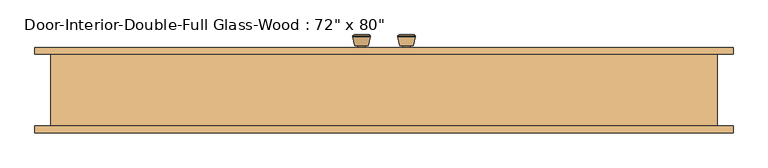
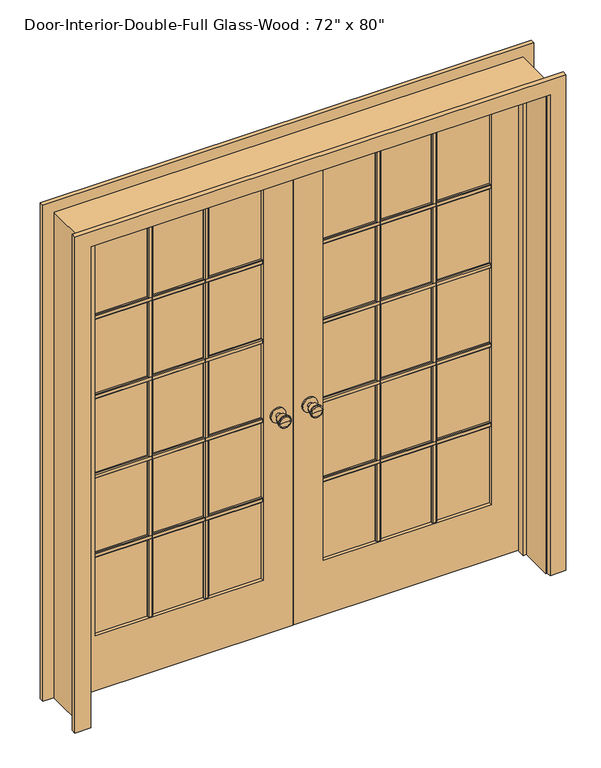
"""IFC4 building model written with IfcOpenShell, lengths in millimetres: door geometry."""

from ifc_helpers import new_model, si_unit, point, frame, frame_2d, origin, place, context, project, spatial, polyline, circle_curve, trimmed, segment, composite_curve, outline, extrude, faceted_brep, source, transform, mapped, element, save
from ifc_brep_helpers import plane_surface, cylinder_surface, revolved_surface, advanced_brep


def door_48c357d2(model_context):
    return source(origin(), model_context, "Body", "SolidModel", [
        advanced_brep(
        [(-63.5, 104.425, 914.4), (-73.5, 104.425, 914.4), (-53.5, 104.425, 914.4), (-83.9758676, 153.425, 914.4), (-63.5, 153.425, 914.4), (-43.0241324, 153.425, 914.4), (-88.5, 151.5971319, 914.4), (-38.5, 151.5971319, 914.4), (-88.5, 148.1334537, 914.4), (-38.5, 148.1334537, 914.4), (-82.136236, 123.425, 914.4), (-44.863764, 123.425, 914.4), (-73.5, 123.425, 914.4), (-53.5, 123.425, 914.4)],
        [
            (0, 1),
            (1, 2, circle_curve(frame((-63.5, 104.425, 914.4), z_axis=(0.0, -1.0, 0.0), x_axis=(1.0, 0.0, 0.0)), 10.0)),
            (2, 0),
            (2, 1, circle_curve(frame((-63.5, 104.425, 914.4), z_axis=(0.0, -1.0, 0.0), x_axis=(1.0, 0.0, 0.0)), 10.0)),
            (3, 4),
            (4, 5),
            (5, 3, circle_curve(frame((-63.5, 153.425, 914.4), z_axis=(0.0, 1.0, 0.0), x_axis=(1.0, 0.0, 0.0)), 20.4758676)),
            (3, 5, circle_curve(frame((-63.5, 153.425, 914.4), z_axis=(0.0, 1.0, 0.0), x_axis=(1.0, 0.0, 0.0)), 20.4758676)),
            (6, 3),
            (5, 7),
            (7, 6, circle_curve(frame((-63.5, 151.5971319, 914.4), z_axis=(0.0, 1.0, 0.0), x_axis=(1.0, 0.0, 0.0)), 25.0)),
            (6, 7, circle_curve(frame((-63.5, 151.5971319, 914.4), z_axis=(0.0, 1.0, 0.0), x_axis=(1.0, 0.0, 0.0)), 25.0)),
            (8, 6),
            (7, 9),
            (9, 8, circle_curve(frame((-63.5, 148.1334537, 914.4), z_axis=(0.0, 1.0, 0.0), x_axis=(1.0, 0.0, 0.0)), 25.0)),
            (8, 9, circle_curve(frame((-63.5, 148.1334537, 914.4), z_axis=(0.0, 1.0, 0.0), x_axis=(1.0, 0.0, 0.0)), 25.0)),
            (10, 8),
            (9, 11),
            (11, 10, circle_curve(frame((-63.5, 123.425, 914.4), z_axis=(0.0, 1.0, 0.0), x_axis=(1.0, 0.0, 0.0)), 18.636236)),
            (10, 11, circle_curve(frame((-63.5, 123.425, 914.4), z_axis=(0.0, 1.0, 0.0), x_axis=(1.0, 0.0, 0.0)), 18.636236)),
            (12, 10),
            (11, 13),
            (13, 12, circle_curve(frame((-63.5, 123.425, 914.4), z_axis=(0.0, 1.0, 0.0), x_axis=(1.0, 0.0, 0.0)), 10.0)),
            (12, 13, circle_curve(frame((-63.5, 123.425, 914.4), z_axis=(0.0, 1.0, 0.0), x_axis=(1.0, 0.0, 0.0)), 10.0)),
            (1, 12),
            (13, 2),
        ],
        [
            plane_surface(frame((-63.5, 104.425, 914.4), z_axis=(0.0, -1.0, 0.0), x_axis=(1.0, 0.0, 0.0))),
            plane_surface(frame((-63.5, 153.425, 914.4), z_axis=(0.0, 1.0, 0.0), x_axis=(1.0, 0.0, 0.0))),
            revolved_surface(polyline([(-43.0241324, 153.425, 914.4), (-38.5, 151.5971319, 914.4)]), (-63.5, 104.425, 914.4), (0.0, -1.0, 0.0)),
            cylinder_surface(frame((-63.5, 104.425, 914.4), z_axis=(0.0, -1.0, 0.0), x_axis=(1.0, 0.0, 0.0)), 25.0),
            revolved_surface(polyline([(-38.5, 148.1334537, 914.4), (-44.863764, 123.425, 914.4)]), (-63.5, 104.425, 914.4), (0.0, -1.0, 0.0)),
            plane_surface(frame((-63.5, 123.425, 914.4), z_axis=(0.0, -1.0, 0.0), x_axis=(1.0, 0.0, 0.0))),
            cylinder_surface(frame((-63.5, 104.425, 914.4), z_axis=(0.0, -1.0, 0.0), x_axis=(1.0, 0.0, 0.0)), 10.0),
        ],
        [
            (0, [[1, 2, 3]]),
            (0, [[-3, 4, -1]]),
            (1, [[5, 6, 7]]),
            (1, [[-6, -5, 8]]),
            (2, [[9, -7, 10, 11]]),
            (2, [[-10, -8, -9, 12]]),
            (3, [[13, -11, 14, 15]]),
            (3, [[-14, -12, -13, 16]]),
            (4, [[17, -15, 18, 19]]),
            (4, [[-18, -16, -17, 20]]),
            (5, [[21, -19, 22, 23]]),
            (5, [[-22, -20, -21, 24]]),
            (6, [[25, -23, 26, -2]]),
            (6, [[-26, -24, -25, -4]]),
        ],
    ),
        extrude(outline(composite_curve([segment(trimmed(circle_curve(frame_2d((914.4, -63.5)), 30.0), [point((914.4, -33.5))], [point((914.4, -93.5))], False, "CARTESIAN"), True, "CONTINUOUS"), segment(trimmed(circle_curve(frame_2d((914.4, -63.5)), 30.0), [point((914.4, -93.5))], [point((914.4, -33.5))], False, "CARTESIAN"), True, "CONTINUOUS")], self_intersect=False)), frame((0.0, 98.425, 0.0), z_axis=(0.0, 1.0, 0.0), x_axis=(0.0, 0.0, 1.0)), (0.0, 0.0, 1.0), 6.0),
        advanced_brep(
        [(-63.5, 57.5, 914.4), (-53.5, 57.5, 914.4), (-73.5, 57.5, 914.4), (-83.9758676, 8.5, 914.4), (-43.0241324, 8.5, 914.4), (-63.5, 8.5, 914.4), (-88.5, 10.3278681, 914.4), (-38.5, 10.3278681, 914.4), (-88.5, 13.7915463, 914.4), (-38.5, 13.7915463, 914.4), (-82.136236, 38.5, 914.4), (-44.863764, 38.5, 914.4), (-73.5, 38.5, 914.4), (-53.5, 38.5, 914.4)],
        [
            (0, 1),
            (1, 2, circle_curve(frame((-63.5, 57.5, 914.4), z_axis=(0.0, 1.0, 0.0), x_axis=(1.0, 0.0, 0.0)), 10.0)),
            (2, 0),
            (2, 1, circle_curve(frame((-63.5, 57.5, 914.4), z_axis=(0.0, 1.0, 0.0), x_axis=(1.0, 0.0, 0.0)), 10.0)),
            (3, 4, circle_curve(frame((-63.5, 8.5, 914.4), z_axis=(0.0, -1.0, 0.0), x_axis=(1.0, 0.0, 0.0)), 20.4758676)),
            (4, 5),
            (5, 3),
            (4, 3, circle_curve(frame((-63.5, 8.5, 914.4), z_axis=(0.0, -1.0, 0.0), x_axis=(1.0, 0.0, 0.0)), 20.4758676)),
            (6, 7, circle_curve(frame((-63.5, 10.3278681, 914.4), z_axis=(0.0, -1.0, 0.0), x_axis=(1.0, 0.0, 0.0)), 25.0)),
            (7, 4),
            (3, 6),
            (7, 6, circle_curve(frame((-63.5, 10.3278681, 914.4), z_axis=(0.0, -1.0, 0.0), x_axis=(1.0, 0.0, 0.0)), 25.0)),
            (8, 9, circle_curve(frame((-63.5, 13.7915463, 914.4), z_axis=(0.0, -1.0, 0.0), x_axis=(1.0, 0.0, 0.0)), 25.0)),
            (9, 7),
            (6, 8),
            (9, 8, circle_curve(frame((-63.5, 13.7915463, 914.4), z_axis=(0.0, -1.0, 0.0), x_axis=(1.0, 0.0, 0.0)), 25.0)),
            (10, 11, circle_curve(frame((-63.5, 38.5, 914.4), z_axis=(0.0, -1.0, 0.0), x_axis=(1.0, 0.0, 0.0)), 18.636236)),
            (11, 9),
            (8, 10),
            (11, 10, circle_curve(frame((-63.5, 38.5, 914.4), z_axis=(0.0, -1.0, 0.0), x_axis=(1.0, 0.0, 0.0)), 18.636236)),
            (12, 13, circle_curve(frame((-63.5, 38.5, 914.4), z_axis=(0.0, -1.0, 0.0), x_axis=(1.0, 0.0, 0.0)), 10.0)),
            (13, 11),
            (10, 12),
            (13, 12, circle_curve(frame((-63.5, 38.5, 914.4), z_axis=(0.0, -1.0, 0.0), x_axis=(1.0, 0.0, 0.0)), 10.0)),
            (1, 13),
            (12, 2),
        ],
        [
            plane_surface(frame((-63.5, 57.5, 914.4), z_axis=(0.0, 1.0, 0.0), x_axis=(1.0, 0.0, 0.0))),
            plane_surface(frame((-63.5, 8.5, 914.4), z_axis=(0.0, -1.0, 0.0), x_axis=(1.0, 0.0, 0.0))),
            revolved_surface(polyline([(-43.0241324, 8.5, 914.4), (-38.5, 10.3278681, 914.4)]), (-63.5, 57.5, 914.4), (0.0, 1.0, 0.0)),
            cylinder_surface(frame((-63.5, 57.5, 914.4), z_axis=(0.0, 1.0, 0.0), x_axis=(1.0, 0.0, 0.0)), 25.0),
            revolved_surface(polyline([(-38.5, 13.7915463, 914.4), (-44.863764, 38.5, 914.4)]), (-63.5, 57.5, 914.4), (0.0, 1.0, 0.0)),
            plane_surface(frame((-63.5, 38.5, 914.4), z_axis=(0.0, 1.0, 0.0), x_axis=(1.0, 0.0, 0.0))),
            cylinder_surface(frame((-63.5, 57.5, 914.4), z_axis=(0.0, 1.0, 0.0), x_axis=(1.0, 0.0, 0.0)), 10.0),
        ],
        [
            (0, [[1, 2, 3]]),
            (0, [[-3, 4, -1]]),
            (1, [[5, 6, 7]]),
            (1, [[8, -7, -6]]),
            (2, [[9, 10, -5, 11]]),
            (2, [[12, -11, -8, -10]]),
            (3, [[13, 14, -9, 15]]),
            (3, [[16, -15, -12, -14]]),
            (4, [[17, 18, -13, 19]]),
            (4, [[20, -19, -16, -18]]),
            (5, [[21, 22, -17, 23]]),
            (5, [[24, -23, -20, -22]]),
            (6, [[-2, 25, -21, 26]]),
            (6, [[-4, -26, -24, -25]]),
        ],
    ),
        extrude(outline(composite_curve([segment(trimmed(circle_curve(frame_2d((914.4, -63.5)), 30.0), [point((914.4, -33.5))], [point((914.4, -93.5))], False, "CARTESIAN"), True, "CONTINUOUS"), segment(trimmed(circle_curve(frame_2d((914.4, -63.5)), 30.0), [point((914.4, -93.5))], [point((914.4, -33.5))], False, "CARTESIAN"), True, "CONTINUOUS")], self_intersect=False)), frame((0.0, 57.5, 0.0), z_axis=(0.0, 1.0, 0.0), x_axis=(0.0, 0.0, 1.0)), (0.0, 0.0, 1.0), 6.0),
        extrude(outline(polyline([(77.47, 1586.23), (77.47, 1567.18), (71.12, 1567.18), (67.945, 1570.355), (67.945, 1583.055), (71.12, 1586.23), (77.47, 1586.23)])), frame((120.65, 0.0, 0.0), z_axis=(1.0, 0.0, 0.0), x_axis=(0.0, 1.0, 0.0)), (0.0, 0.0, 1.0), 673.1),
        extrude(outline(polyline([(77.47, 1249.9975), (77.47, 1230.9475), (71.12, 1230.9475), (67.945, 1234.1225), (67.945, 1246.8225), (71.12, 1249.9975), (77.47, 1249.9975)])), frame((120.65, 0.0, 0.0), z_axis=(1.0, 0.0, 0.0), x_axis=(0.0, 1.0, 0.0)), (0.0, 0.0, 1.0), 673.1),
        extrude(outline(polyline([(77.47, 913.765), (77.47, 894.715), (71.12, 894.715), (67.945, 897.89), (67.945, 910.59), (71.12, 913.765), (77.47, 913.765)])), frame((120.65, 0.0, 0.0), z_axis=(1.0, 0.0, 0.0), x_axis=(0.0, 1.0, 0.0)), (0.0, 0.0, 1.0), 673.1),
        extrude(outline(polyline([(77.47, 577.5325), (77.47, 558.4825), (71.12, 558.4825), (67.945, 561.6575), (67.945, 574.3575), (71.12, 577.5325), (77.47, 577.5325)])), frame((120.65, 0.0, 0.0), z_axis=(1.0, 0.0, 0.0), x_axis=(0.0, 1.0, 0.0)), (0.0, 0.0, 1.0), 673.1),
        extrude(outline(polyline([(559.8583333, 77.47), (578.9083333, 77.47), (578.9083333, 71.12), (575.7333333, 67.945), (563.0333333, 67.945), (559.8583333, 71.12), (559.8583333, 77.47)])), frame((0.0, 0.0, 231.775), z_axis=(0.0, 0.0, 1.0), x_axis=(1.0, 0.0, 0.0)), (0.0, 0.0, 1.0), 1681.1625),
        extrude(outline(polyline([(335.4916667, 77.47), (354.5416667, 77.47), (354.5416667, 71.12), (351.3666667, 67.945), (338.6666667, 67.945), (335.4916667, 71.12), (335.4916667, 77.47)])), frame((0.0, 0.0, 231.775), z_axis=(0.0, 0.0, 1.0), x_axis=(1.0, 0.0, 0.0)), (0.0, 0.0, 1.0), 1681.1625),
        extrude(outline(polyline([(84.455, 1586.23), (90.805, 1586.23), (93.98, 1583.055), (93.98, 1570.355), (90.805, 1567.18), (84.455, 1567.18), (84.455, 1586.23)])), frame((-793.75, 0.0, 0.0), z_axis=(1.0, 0.0, 0.0), x_axis=(0.0, 1.0, 0.0)), (0.0, 0.0, 1.0), 673.1),
        extrude(outline(polyline([(84.455, 1249.9975), (90.805, 1249.9975), (93.98, 1246.8225), (93.98, 1234.1225), (90.805, 1230.9475), (84.455, 1230.9475), (84.455, 1249.9975)])), frame((-793.75, 0.0, 0.0), z_axis=(1.0, 0.0, 0.0), x_axis=(0.0, 1.0, 0.0)), (0.0, 0.0, 1.0), 673.1),
        extrude(outline(polyline([(84.455, 913.765), (90.805, 913.765), (93.98, 910.59), (93.98, 897.89), (90.805, 894.715), (84.455, 894.715), (84.455, 913.765)])), frame((-793.75, 0.0, 0.0), z_axis=(1.0, 0.0, 0.0), x_axis=(0.0, 1.0, 0.0)), (0.0, 0.0, 1.0), 673.1),
        extrude(outline(polyline([(84.455, 577.5325), (90.805, 577.5325), (93.98, 574.3575), (93.98, 561.6575), (90.805, 558.4825), (84.455, 558.4825), (84.455, 577.5325)])), frame((-793.75, 0.0, 0.0), z_axis=(1.0, 0.0, 0.0), x_axis=(0.0, 1.0, 0.0)), (0.0, 0.0, 1.0), 673.1),
        extrude(outline(polyline([(-354.5416667, 84.455), (-354.5416667, 90.805), (-351.3666667, 93.98), (-338.6666667, 93.98), (-335.4916667, 90.805), (-335.4916667, 84.455), (-354.5416667, 84.455)])), frame((0.0, 0.0, 231.775), z_axis=(0.0, 0.0, 1.0), x_axis=(1.0, 0.0, 0.0)), (0.0, 0.0, 1.0), 1681.1625),
        extrude(outline(polyline([(-578.9083333, 84.455), (-578.9083333, 90.805), (-575.7333333, 93.98), (-563.0333333, 93.98), (-559.8583333, 90.805), (-559.8583333, 84.455), (-578.9083333, 84.455)])), frame((0.0, 0.0, 231.775), z_axis=(0.0, 0.0, 1.0), x_axis=(1.0, 0.0, 0.0)), (0.0, 0.0, 1.0), 1681.1625),
        extrude(outline(polyline([(84.455, 1586.23), (90.805, 1586.23), (93.98, 1583.055), (93.98, 1570.355), (90.805, 1567.18), (84.455, 1567.18), (84.455, 1586.23)])), frame((120.65, 0.0, 0.0), z_axis=(1.0, 0.0, 0.0), x_axis=(0.0, 1.0, 0.0)), (0.0, 0.0, 1.0), 673.1),
        extrude(outline(polyline([(84.455, 1249.9975), (90.805, 1249.9975), (93.98, 1246.8225), (93.98, 1234.1225), (90.805, 1230.9475), (84.455, 1230.9475), (84.455, 1249.9975)])), frame((120.65, 0.0, 0.0), z_axis=(1.0, 0.0, 0.0), x_axis=(0.0, 1.0, 0.0)), (0.0, 0.0, 1.0), 673.1),
        extrude(outline(polyline([(84.455, 913.765), (90.805, 913.765), (93.98, 910.59), (93.98, 897.89), (90.805, 894.715), (84.455, 894.715), (84.455, 913.765)])), frame((120.65, 0.0, 0.0), z_axis=(1.0, 0.0, 0.0), x_axis=(0.0, 1.0, 0.0)), (0.0, 0.0, 1.0), 673.1),
        extrude(outline(polyline([(84.455, 577.5325), (90.805, 577.5325), (93.98, 574.3575), (93.98, 561.6575), (90.805, 558.4825), (84.455, 558.4825), (84.455, 577.5325)])), frame((120.65, 0.0, 0.0), z_axis=(1.0, 0.0, 0.0), x_axis=(0.0, 1.0, 0.0)), (0.0, 0.0, 1.0), 673.1),
        extrude(outline(polyline([(559.8583333, 84.455), (559.8583333, 90.805), (563.0333333, 93.98), (575.7333333, 93.98), (578.9083333, 90.805), (578.9083333, 84.455), (559.8583333, 84.455)])), frame((0.0, 0.0, 231.775), z_axis=(0.0, 0.0, 1.0), x_axis=(1.0, 0.0, 0.0)), (0.0, 0.0, 1.0), 1681.1625),
        extrude(outline(polyline([(335.4916667, 84.455), (335.4916667, 90.805), (338.6666667, 93.98), (351.3666667, 93.98), (354.5416667, 90.805), (354.5416667, 84.455), (335.4916667, 84.455)])), frame((0.0, 0.0, 231.775), z_axis=(0.0, 0.0, 1.0), x_axis=(1.0, 0.0, 0.0)), (0.0, 0.0, 1.0), 1681.1625),
        extrude(outline(polyline([(77.47, 1586.23), (77.47, 1567.18), (71.12, 1567.18), (67.945, 1570.355), (67.945, 1583.055), (71.12, 1586.23), (77.47, 1586.23)])), frame((-793.75, 0.0, 0.0), z_axis=(1.0, 0.0, 0.0), x_axis=(0.0, 1.0, 0.0)), (0.0, 0.0, 1.0), 673.1),
        extrude(outline(polyline([(77.47, 1249.9975), (77.47, 1230.9475), (71.12, 1230.9475), (67.945, 1234.1225), (67.945, 1246.8225), (71.12, 1249.9975), (77.47, 1249.9975)])), frame((-793.75, 0.0, 0.0), z_axis=(1.0, 0.0, 0.0), x_axis=(0.0, 1.0, 0.0)), (0.0, 0.0, 1.0), 673.1),
        extrude(outline(polyline([(77.47, 913.765), (77.47, 894.715), (71.12, 894.715), (67.945, 897.89), (67.945, 910.59), (71.12, 913.765), (77.47, 913.765)])), frame((-793.75, 0.0, 0.0), z_axis=(1.0, 0.0, 0.0), x_axis=(0.0, 1.0, 0.0)), (0.0, 0.0, 1.0), 673.1),
        extrude(outline(polyline([(77.47, 577.5325), (77.47, 558.4825), (71.12, 558.4825), (67.945, 561.6575), (67.945, 574.3575), (71.12, 577.5325), (77.47, 577.5325)])), frame((-793.75, 0.0, 0.0), z_axis=(1.0, 0.0, 0.0), x_axis=(0.0, 1.0, 0.0)), (0.0, 0.0, 1.0), 673.1),
        extrude(outline(polyline([(-354.5416667, 77.47), (-335.4916667, 77.47), (-335.4916667, 71.12), (-338.6666667, 67.945), (-351.3666667, 67.945), (-354.5416667, 71.12), (-354.5416667, 77.47)])), frame((0.0, 0.0, 231.775), z_axis=(0.0, 0.0, 1.0), x_axis=(1.0, 0.0, 0.0)), (0.0, 0.0, 1.0), 1681.1625),
        extrude(outline(polyline([(-578.9083333, 77.47), (-559.8583333, 77.47), (-559.8583333, 71.12), (-563.0333333, 67.945), (-575.7333333, 67.945), (-578.9083333, 71.12), (-578.9083333, 77.47)])), frame((0.0, 0.0, 231.775), z_axis=(0.0, 0.0, 1.0), x_axis=(1.0, 0.0, 0.0)), (0.0, 0.0, 1.0), 1681.1625),
        advanced_brep(
        [(63.5, 57.5, 914.4), (73.5, 57.5, 914.4), (53.5, 57.5, 914.4), (83.9758676, 8.5, 914.4), (63.5, 8.5, 914.4), (43.0241324, 8.5, 914.4), (88.5, 10.3278681, 914.4), (38.5, 10.3278681, 914.4), (88.5, 13.7915463, 914.4), (38.5, 13.7915463, 914.4), (82.136236, 38.5, 914.4), (44.863764, 38.5, 914.4), (73.5, 38.5, 914.4), (53.5, 38.5, 914.4)],
        [
            (0, 1),
            (1, 2, circle_curve(frame((63.5, 57.5, 914.4), z_axis=(0.0, 1.0, 0.0), x_axis=(-1.0, 0.0, 0.0)), 10.0)),
            (2, 0),
            (2, 1, circle_curve(frame((63.5, 57.5, 914.4), z_axis=(0.0, 1.0, 0.0), x_axis=(-1.0, 0.0, 0.0)), 10.0)),
            (3, 4),
            (4, 5),
            (5, 3, circle_curve(frame((63.5, 8.5, 914.4), z_axis=(0.0, -1.0, 0.0), x_axis=(-1.0, 0.0, 0.0)), 20.4758676)),
            (3, 5, circle_curve(frame((63.5, 8.5, 914.4), z_axis=(0.0, -1.0, 0.0), x_axis=(-1.0, 0.0, 0.0)), 20.4758676)),
            (6, 3),
            (5, 7),
            (7, 6, circle_curve(frame((63.5, 10.3278681, 914.4), z_axis=(0.0, -1.0, 0.0), x_axis=(-1.0, 0.0, 0.0)), 25.0)),
            (6, 7, circle_curve(frame((63.5, 10.3278681, 914.4), z_axis=(0.0, -1.0, 0.0), x_axis=(-1.0, 0.0, 0.0)), 25.0)),
            (8, 6),
            (7, 9),
            (9, 8, circle_curve(frame((63.5, 13.7915463, 914.4), z_axis=(0.0, -1.0, 0.0), x_axis=(-1.0, 0.0, 0.0)), 25.0)),
            (8, 9, circle_curve(frame((63.5, 13.7915463, 914.4), z_axis=(0.0, -1.0, 0.0), x_axis=(-1.0, 0.0, 0.0)), 25.0)),
            (10, 8),
            (9, 11),
            (11, 10, circle_curve(frame((63.5, 38.5, 914.4), z_axis=(0.0, -1.0, 0.0), x_axis=(-1.0, 0.0, 0.0)), 18.636236)),
            (10, 11, circle_curve(frame((63.5, 38.5, 914.4), z_axis=(0.0, -1.0, 0.0), x_axis=(-1.0, 0.0, 0.0)), 18.636236)),
            (12, 10),
            (11, 13),
            (13, 12, circle_curve(frame((63.5, 38.5, 914.4), z_axis=(0.0, -1.0, 0.0), x_axis=(-1.0, 0.0, 0.0)), 10.0)),
            (12, 13, circle_curve(frame((63.5, 38.5, 914.4), z_axis=(0.0, -1.0, 0.0), x_axis=(-1.0, 0.0, 0.0)), 10.0)),
            (1, 12),
            (13, 2),
        ],
        [
            plane_surface(frame((63.5, 57.5, 914.4), z_axis=(0.0, 1.0, 0.0), x_axis=(-1.0, 0.0, 0.0))),
            plane_surface(frame((63.5, 8.5, 914.4), z_axis=(0.0, -1.0, 0.0), x_axis=(-1.0, 0.0, 0.0))),
            revolved_surface(polyline([(43.0241324, 8.5, 914.4), (38.5, 10.3278681, 914.4)]), (63.5, 57.5, 914.4), (0.0, 1.0, 0.0)),
            cylinder_surface(frame((63.5, 57.5, 914.4), z_axis=(0.0, 1.0, 0.0), x_axis=(-1.0, 0.0, 0.0)), 25.0),
            revolved_surface(polyline([(38.5, 13.7915463, 914.4), (44.863764, 38.5, 914.4)]), (63.5, 57.5, 914.4), (0.0, 1.0, 0.0)),
            plane_surface(frame((63.5, 38.5, 914.4), z_axis=(0.0, 1.0, 0.0), x_axis=(-1.0, 0.0, 0.0))),
            cylinder_surface(frame((63.5, 57.5, 914.4), z_axis=(0.0, 1.0, 0.0), x_axis=(-1.0, 0.0, 0.0)), 10.0),
        ],
        [
            (0, [[1, 2, 3]]),
            (0, [[-3, 4, -1]]),
            (1, [[5, 6, 7]]),
            (1, [[-6, -5, 8]]),
            (2, [[9, -7, 10, 11]]),
            (2, [[-10, -8, -9, 12]]),
            (3, [[13, -11, 14, 15]]),
            (3, [[-14, -12, -13, 16]]),
            (4, [[17, -15, 18, 19]]),
            (4, [[-18, -16, -17, 20]]),
            (5, [[21, -19, 22, 23]]),
            (5, [[-22, -20, -21, 24]]),
            (6, [[25, -23, 26, -2]]),
            (6, [[-26, -24, -25, -4]]),
        ],
    ),
        extrude(outline(composite_curve([segment(trimmed(circle_curve(frame_2d((914.4, 63.5)), 30.0), [point((914.4, 33.5))], [point((914.4, 93.5))], False, "CARTESIAN"), True, "CONTINUOUS"), segment(trimmed(circle_curve(frame_2d((914.4, 63.5)), 30.0), [point((914.4, 93.5))], [point((914.4, 33.5))], False, "CARTESIAN"), True, "CONTINUOUS")], self_intersect=False)), frame((0.0, 57.5, 0.0), z_axis=(0.0, 1.0, 0.0), x_axis=(0.0, 0.0, 1.0)), (0.0, 0.0, 1.0), 6.0),
        advanced_brep(
        [(63.5, 104.425, 914.4), (53.5, 104.425, 914.4), (73.5, 104.425, 914.4), (83.9758676, 153.425, 914.4), (43.0241324, 153.425, 914.4), (63.5, 153.425, 914.4), (88.5, 151.5971319, 914.4), (38.5, 151.5971319, 914.4), (88.5, 148.1334537, 914.4), (38.5, 148.1334537, 914.4), (82.136236, 123.425, 914.4), (44.863764, 123.425, 914.4), (73.5, 123.425, 914.4), (53.5, 123.425, 914.4)],
        [
            (0, 1),
            (1, 2, circle_curve(frame((63.5, 104.425, 914.4), z_axis=(0.0, -1.0, 0.0), x_axis=(-1.0, 0.0, 0.0)), 10.0)),
            (2, 0),
            (2, 1, circle_curve(frame((63.5, 104.425, 914.4), z_axis=(0.0, -1.0, 0.0), x_axis=(-1.0, 0.0, 0.0)), 10.0)),
            (3, 4, circle_curve(frame((63.5, 153.425, 914.4), z_axis=(0.0, 1.0, 0.0), x_axis=(-1.0, 0.0, 0.0)), 20.4758676)),
            (4, 5),
            (5, 3),
            (4, 3, circle_curve(frame((63.5, 153.425, 914.4), z_axis=(0.0, 1.0, 0.0), x_axis=(-1.0, 0.0, 0.0)), 20.4758676)),
            (6, 7, circle_curve(frame((63.5, 151.5971319, 914.4), z_axis=(0.0, 1.0, 0.0), x_axis=(-1.0, 0.0, 0.0)), 25.0)),
            (7, 4),
            (3, 6),
            (7, 6, circle_curve(frame((63.5, 151.5971319, 914.4), z_axis=(0.0, 1.0, 0.0), x_axis=(-1.0, 0.0, 0.0)), 25.0)),
            (8, 9, circle_curve(frame((63.5, 148.1334537, 914.4), z_axis=(0.0, 1.0, 0.0), x_axis=(-1.0, 0.0, 0.0)), 25.0)),
            (9, 7),
            (6, 8),
            (9, 8, circle_curve(frame((63.5, 148.1334537, 914.4), z_axis=(0.0, 1.0, 0.0), x_axis=(-1.0, 0.0, 0.0)), 25.0)),
            (10, 11, circle_curve(frame((63.5, 123.425, 914.4), z_axis=(0.0, 1.0, 0.0), x_axis=(-1.0, 0.0, 0.0)), 18.636236)),
            (11, 9),
            (8, 10),
            (11, 10, circle_curve(frame((63.5, 123.425, 914.4), z_axis=(0.0, 1.0, 0.0), x_axis=(-1.0, 0.0, 0.0)), 18.636236)),
            (12, 13, circle_curve(frame((63.5, 123.425, 914.4), z_axis=(0.0, 1.0, 0.0), x_axis=(-1.0, 0.0, 0.0)), 10.0)),
            (13, 11),
            (10, 12),
            (13, 12, circle_curve(frame((63.5, 123.425, 914.4), z_axis=(0.0, 1.0, 0.0), x_axis=(-1.0, 0.0, 0.0)), 10.0)),
            (1, 13),
            (12, 2),
        ],
        [
            plane_surface(frame((63.5, 104.425, 914.4), z_axis=(0.0, -1.0, 0.0), x_axis=(-1.0, 0.0, 0.0))),
            plane_surface(frame((63.5, 153.425, 914.4), z_axis=(0.0, 1.0, 0.0), x_axis=(-1.0, 0.0, 0.0))),
            revolved_surface(polyline([(43.0241324, 153.425, 914.4), (38.5, 151.5971319, 914.4)]), (63.5, 104.425, 914.4), (0.0, -1.0, 0.0)),
            cylinder_surface(frame((63.5, 104.425, 914.4), z_axis=(0.0, -1.0, 0.0), x_axis=(-1.0, 0.0, 0.0)), 25.0),
            revolved_surface(polyline([(38.5, 148.1334537, 914.4), (44.863764, 123.425, 914.4)]), (63.5, 104.425, 914.4), (0.0, -1.0, 0.0)),
            plane_surface(frame((63.5, 123.425, 914.4), z_axis=(0.0, -1.0, 0.0), x_axis=(-1.0, 0.0, 0.0))),
            cylinder_surface(frame((63.5, 104.425, 914.4), z_axis=(0.0, -1.0, 0.0), x_axis=(-1.0, 0.0, 0.0)), 10.0),
        ],
        [
            (0, [[1, 2, 3]]),
            (0, [[-3, 4, -1]]),
            (1, [[5, 6, 7]]),
            (1, [[8, -7, -6]]),
            (2, [[9, 10, -5, 11]]),
            (2, [[12, -11, -8, -10]]),
            (3, [[13, 14, -9, 15]]),
            (3, [[16, -15, -12, -14]]),
            (4, [[17, 18, -13, 19]]),
            (4, [[20, -19, -16, -18]]),
            (5, [[21, 22, -17, 23]]),
            (5, [[24, -23, -20, -22]]),
            (6, [[-2, 25, -21, 26]]),
            (6, [[-4, -26, -24, -25]]),
        ],
    ),
        extrude(outline(composite_curve([segment(trimmed(circle_curve(frame_2d((914.4, 63.5)), 30.0), [point((914.4, 33.5))], [point((914.4, 93.5))], False, "CARTESIAN"), True, "CONTINUOUS"), segment(trimmed(circle_curve(frame_2d((914.4, 63.5)), 30.0), [point((914.4, 93.5))], [point((914.4, 33.5))], False, "CARTESIAN"), True, "CONTINUOUS")], self_intersect=False)), frame((0.0, 98.425, 0.0), z_axis=(0.0, 1.0, 0.0), x_axis=(0.0, 0.0, 1.0)), (0.0, 0.0, 1.0), 6.0),
        extrude(outline(polyline([(0.0, 920.75), (0.0, 984.25), (2101.85, 984.25), (2101.85, -984.25), (0.0, -984.25), (0.0, -920.75), (2038.35, -920.75), (2038.35, 920.75), (0.0, 920.75)])), frame((0.0, 98.425, 0.0), z_axis=(0.0, 1.0, 0.0), x_axis=(0.0, 0.0, 1.0)), (0.0, 0.0, 1.0), 19.05),
        extrude(outline(polyline([(0.0, 920.75), (0.0, 984.25), (2101.85, 984.25), (2101.85, -984.25), (0.0, -984.25), (0.0, -920.75), (2038.35, -920.75), (2038.35, 920.75), (0.0, 920.75)])), frame((0.0, -123.825, 0.0), z_axis=(0.0, 1.0, 0.0), x_axis=(0.0, 0.0, 1.0)), (0.0, 0.0, 1.0), 19.05),
        extrude(outline(polyline([(2032.0, -914.4), (0.0, -914.4), (0.0, -1.6019111), (2032.0, -1.6019111), (2032.0, -914.4)]), holes=[polyline([(231.775, -793.75), (1912.9375, -793.75), (1912.9375, -120.65), (231.775, -120.65), (231.775, -793.75)])]), frame((0.0, 63.5, 0.0), z_axis=(0.0, 1.0, 0.0), x_axis=(0.0, 0.0, 1.0)), (0.0, 0.0, 1.0), 34.925),
        extrude(outline(polyline([(0.0, 914.4), (2032.0, 914.4), (2032.0, 1.5875), (0.0, 1.5875), (0.0, 914.4)]), holes=[polyline([(1912.9375, 120.65), (1912.9375, 793.75), (231.775, 793.75), (231.775, 120.65), (1912.9375, 120.65)])]), frame((0.0, 63.5, 0.0), z_axis=(0.0, 1.0, 0.0), x_axis=(0.0, 0.0, 1.0)), (0.0, 0.0, 1.0), 34.925),
        faceted_brep([(939.8, 98.425, 0.0), (939.8, -104.775, 0.0), (914.4, -104.775, 0.0), (914.4, 28.575, 0.0), (901.7, 28.575, 0.0), (901.7, 63.5, 0.0), (914.4, 63.5, 0.0), (914.4, 98.425, 0.0), (939.8, 98.425, 2057.4), (939.8, -104.775, 2057.4), (-939.8, -104.775, 2057.4), (-939.8, -104.775, 0.0), (-914.4, -104.775, 0.0), (-914.4, -104.775, 2032.0), (914.4, -104.775, 2032.0), (914.4, 28.575, 2032.0), (-914.4, 28.575, 2032.0), (-914.4, 28.575, 0.0), (-901.7, 28.575, 0.0), (-901.7, 28.575, 2019.3), (901.7, 28.575, 2019.3), (901.7, 63.5, 2019.3), (1.5875, 63.5, 2019.3), (-1.6019111, 63.5, 2019.3), (-901.7, 63.5, 2019.3), (-901.7, 63.5, 0.0), (-914.4, 63.5, 0.0), (-914.4, 63.5, 2032.0), (-1.6019111, 63.5, 2032.0), (1.5875, 63.5, 2032.0), (914.4, 63.5, 2032.0), (914.4, 98.425, 2032.0), (1.5875, 98.425, 2032.0), (-1.6019111, 98.425, 2032.0), (-914.4, 98.425, 2032.0), (-914.4, 98.425, 0.0), (-939.8, 98.425, 0.0), (-939.8, 98.425, 2057.4)], [[[0, 1, 2, 3, 4, 5, 6, 7]], [[1, 0, 8, 9]], [[2, 1, 9, 10, 11, 12, 13, 14]], [[3, 2, 14, 15]], [[4, 3, 15, 16, 17, 18, 19, 20]], [[5, 4, 20, 21]], [[6, 5, 21, 22, 23, 24, 25, 26, 27, 28, 29, 30]], [[7, 6, 30, 31]], [[0, 7, 31, 32, 33, 34, 35, 36, 37, 8]], [[9, 8, 37, 10]], [[14, 13, 16, 15]], [[20, 19, 24, 23, 22, 21]], [[31, 30, 29, 28, 27, 34, 33, 32]], [[12, 11, 36, 35, 26, 25, 18, 17]], [[11, 10, 37, 36]], [[13, 12, 17, 16]], [[19, 18, 25, 24]], [[27, 26, 35, 34]]]),
        extrude(outline(polyline([(793.75, 77.47), (120.65, 77.47), (120.65, 84.455), (793.75, 84.455), (793.75, 77.47)])), frame((0.0, 0.0, 231.775), z_axis=(0.0, 0.0, 1.0), x_axis=(1.0, 0.0, 0.0)), (0.0, 0.0, 1.0), 1681.1625),
        extrude(outline(polyline([(-120.65, 77.47), (-793.75, 77.47), (-793.75, 84.455), (-120.65, 84.455), (-120.65, 77.47)])), frame((0.0, 0.0, 231.775), z_axis=(0.0, 0.0, 1.0), x_axis=(1.0, 0.0, 0.0)), (0.0, 0.0, 1.0), 1681.1625),
    ])


if __name__ == "__main__":
    model = new_model("IFC4")
    model_context = context("Model", 3, world=origin())
    ifc_project = project(units=[si_unit("LENGTHUNIT", "METRE", prefix="MILLI")], contexts=[model_context])
    site = spatial("IfcSite", under=ifc_project)
    building = spatial("IfcBuilding", under=site)
    placement = place(None, origin())
    door_shape = door_48c357d2(model_context)
    element("IfcDoor", 1, ObjectType="Door-Interior-Double-Full Glass-Wood : 72\" x 80\"", at=placement, inside=building, context=model_context, shape_type="MappedRepresentation", body=[
        mapped(door_shape, transform((0.0, 0.0, 0.0), x_axis=(1.0, 0.0, 0.0), y_axis=(0.0, 1.0, 0.0), z_axis=(0.0, 0.0, 1.0))),
    ])
    save(model, "model.ifc")

# Revit data of these elements
# Type "Door-Interior-Double-Full Glass-Wood : 72\" x 80\""
#   Type Mark = "8"
#   Assembly Code = "C1020300"
#   Analytic Construction = "French door, wood frame with single glass"
#   Top Rail = 0' - 4 11/16"
#   Thickness = 0' - 1 3/8"
#   Thermal Resistance (R) = 1.0696 (h·ft²·°F)/BTU
#   Swing Angle [instance default] = 90.00°
#   Stiles = 0' - 4 3/4"
#   Rough Width = 6' - 2"
#   Rough Height = 6' - 9"
#   Panel Width = 3' - 0"
#   Height = 6' - 8"
#   Width = 6' - 0"
#   Heat Transfer Coefficient (U) = 0.9350 BTU/(h·ft²·°F)
#   Bottom Rail = 0' - 9 1/8"
#   Show Grill [instance default] = yes
#   Trim Material = Cherry
#   Panel Material = Cherry
#   Frame Material = Cherry
#   Door Handle Material = Aluminum
#   Visual Light Transmittance = 0
#   Solar Heat Gain Coefficient = 0
#   Wall Closure = (empty or 0)
#   Function = (empty or 0)
# Element 1 (IfcDoor, "Door-Interior-Double-Full Glass-Wood : 72\" x 80\"")
#   Materials on its faces: "Cherry", "Aluminum", "Glass"
# Materials
#   "Cherry": class "Wood", colour RGB 226 177 128, transparency 0, Description = "Prunus Serotina", Cost = 0
#   "Aluminum": class "Metal", colour RGB 247 247 247, transparency 0, Description = "Aluminum 6061", Cost = 0
#   "Glass": class "Glass", colour RGB 0 128 192, transparency 0.75, Description = "Soda Lime Glass", Cost = 0
